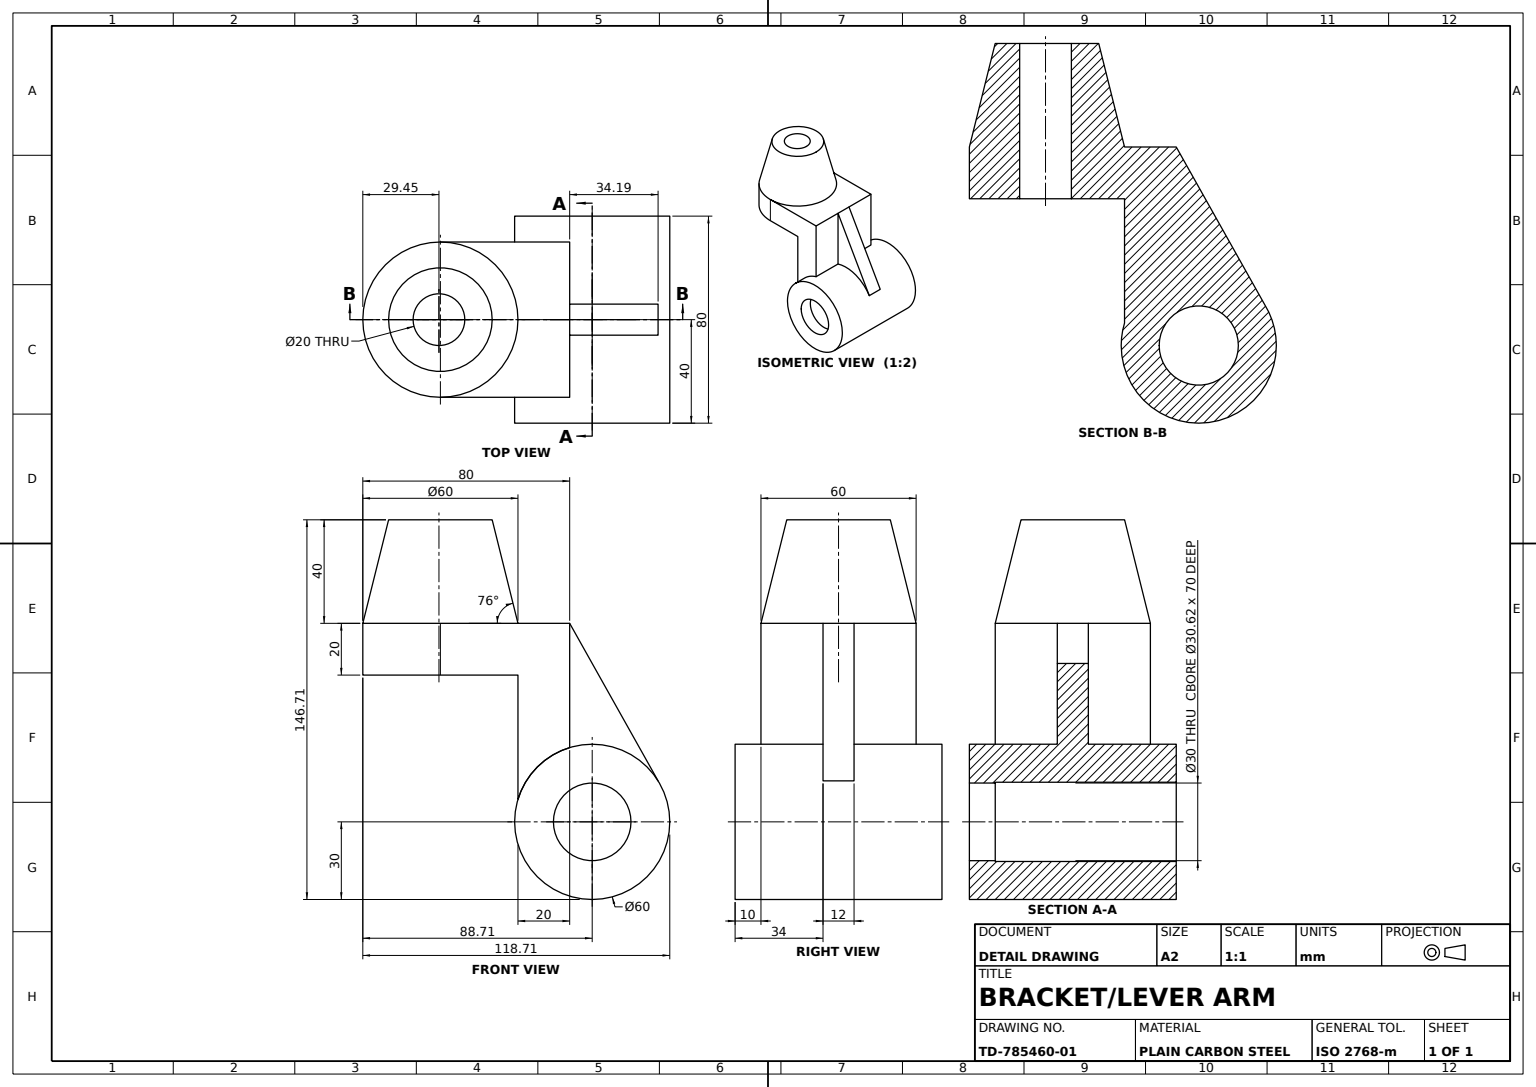
SolidWorks part; units mm, degrees
material "Plain Carbon Steel"
ref_plane "Front Plane" through (0, 0, 0) normal (0, 0, 1) x (1, 0, 0)
ref_plane "Top Plane" through (0, 0, 0) normal (0, 1, 0) x (1, 0, 0)
ref_plane "Right Plane" through (0, 0, 0) normal (1, 0, 0) x (0, 0, -1)
sketch "Base Cylinder Sketch" plane through (0, 0, 0) normal (0, 0, 1) x (1, 0, 0)
  circle A0 centre (0, 0) radius 30
  circle A1 centre (0, 0) radius 15
  dimension "D1" = 60
  dimension "D2" = 30
extrude "Base Cylinder Ø60" add sketch "Base Cylinder Sketch" along normal mid plane 40
sketch "Support Arm Sketch" plane through (0, 0, 0) normal (0, 0, 1) x (1, 0, 0)
  line L0 (-28.7083, 8.7083) -> (-28.7083, 56.7083)
  line L1 (-8.7083, 76.7083) -> (-8.7083, 28.7083)
  line L2 (-8.7083, 76.7083) -> (-88.7083, 76.7083)
  line L3 (-88.7083, 76.7083) -> (-88.7083, 56.7083)
  line L4 (-88.7083, 56.7083) -> (-28.7083, 56.7083)
  circle A0 centre (0, 0) radius 30 construction
  circle A1 centre (0, 0) radius 30
  dimension "D1" = 48
  dimension "D2" = 48
  dimension "D3" = 20
  dimension "D4" = 20
  dimension "D5" = 80
extrude "Support Arm" add sketch "Support Arm Sketch" along normal mid plane 60 contours A1 L1 L2 L3 L4 L0
sketch "Hub Boss A Sketch" plane through (0, 0, 20) normal (0, 0, 1) x (1, 0, 0)
  circle A0 centre (0, 0) radius 30
  dimension "D1" = 60
extrude "Hub Boss A" add sketch "Hub Boss A Sketch" along normal mid plane 20
sketch "Hub Boss B Sketch" plane through (0, 0, -20) normal (0, 0, -1) x (-1, 0, 0)
  circle A0 centre (0, 0) radius 30
  dimension "D1" = 60
extrude "Hub Boss B" add sketch "Hub Boss B Sketch" along normal mid plane 20
sketch "Arm Pad Sketch" plane through (0, 0, 30) normal (0, 0, 1) x (1, 0, 0)
  circle A0 centre (0, 0) radius 30
  circle A1 centre (0, 0) radius 15
  dimension "D1" = 30
  dimension "D2" = 60
extrude "Arm Pad" add sketch "Arm Pad Sketch" along normal mid plane 20
sketch "Arm Boss Sketch" plane through (0, 0, -30) normal (0, 0, -1) x (-1, 0, 0)
  circle A0 centre (0, 0) radius 30
  dimension "D1" = 60
extrude "Arm Boss" add sketch "Arm Boss Sketch" along normal mid plane 20
sketch "Rib Reference Sketch" plane through (0, 0, 40) normal (0, 0, 1) x (1, 0, 0)
  circle A0 centre (0, 0) radius 30 construction
  circle A1 centre (0, 0) radius 30
sketch "Rib Profile Sketch" plane through (0, 0, 0) normal (0, 0, 1) x (1, 0, 0)
  line L0 (-8.7083, 76.7083) -> (-8.7083, 28.7083)
  line L1 (-8.7083, 76.7083) -> (-8.7083, 28.7083) construction
  line L2 (-8.7083, 76.7083) -> (25.4775, 15.8398)
  circle A0 centre (0, 0) radius 30 construction
  arc A1 (-8.7083, 28.7083) -> (25.4775, 15.8398) centre (0, 0) cw
  dimension "D1" = 34.1858
extrude "Support Rib 12mm" add sketch "Rib Profile Sketch" along normal mid plane 12
sketch "Arm Pocket Sketch" plane through (0, 76.7083, 0) normal (0, 1, 0) x (1, 0, 0)
  line L2 (-58.7083, -30) -> (-88.7083, -30)
  line L3 (-88.7083, -30) -> (-88.7083, 30)
  line L4 (-88.7083, 30) -> (-58.7083, 30)
  arc A0 (-58.7083, 30) -> (-58.7083, -30) centre (-58.7083, 0) ccw
  line M6 (-8.7083, 30) -> (-88.7083, 30)
  line M7 (-88.7083, 30) -> (-88.7083, -30)
  line M8 (-88.7083, -30) -> (-8.7083, -30)
extrude "Arm Pocket Cut" cut sketch "Arm Pocket Sketch" against normal blind 40 contours A0 L3 M8 | A0 M6 M7
sketch "Tapered Boss Sketch" plane through (0, 76.7083, 0) normal (0, 1, 0) x (1, 0, 0)
  circle A0 centre (-58.7083, 0) radius 30
  dimension "D1" = 60
extrude "Tapered Boss 14deg Draft" add sketch "Tapered Boss Sketch" along normal blind 40 draft 14
sketch "Boss Hole Sketch" plane through (0, 116.7083, 0) normal (0, 1, 0) x (1, 0, 0)
  circle A0 centre (-59.2629, 0) radius 10
  dimension "D1" = 20
  dimension "D2" = 59.2629
extrude "Boss Hole Ø20" cut sketch "Boss Hole Sketch" against normal through all
sketch "Cylinder Bore Sketch" plane through (0, 0, 30) normal (0, 0, 1) x (1, 0, 0)
  circle A0 centre (0, 0) radius 15.3089
  dimension "D1" = 30.6179
extrude "Cylinder Bore" cut sketch "Cylinder Bore Sketch" against normal through all
